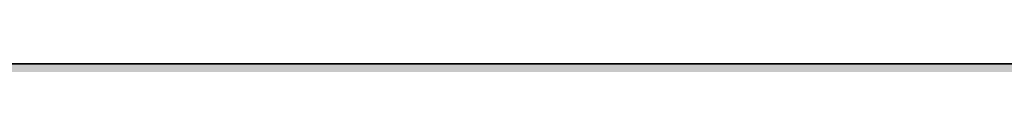
# Model space of a CAD drawing. Units: inches. Extents: x 2091 to 2899, y 967 to 2217.
# Tile 82 of 256: x 2245.941 to 2249.731, y 1099.919 to 1099.919. Entities that reach past the tile are written whole.
import ezdxf

# ---------------------------------------------------------------- set-up
doc = ezdxf.new("R2010")
doc.units = ezdxf.units.IN
doc.layers.add('A-WALL-PATT', color=141, linetype='Continuous', lineweight=13, true_color=0xadddf7)
doc.layers.add('L-SITE-WALL', color=7, linetype='Continuous', lineweight=35)

msp = doc.modelspace()

# ---------------------------------------------------------------- hatches: boundary and pattern name
at = {"layer": 'A-WALL-PATT'}
h = msp.add_hatch(color=256, dxfattribs=at)
h.dxf.hatch_style = 1
h.paths.add_polyline_path([(2212.1436, 1941.4191), (2387.6436, 1941.4191), (2387.6436, 1824.4191), (2392.1436, 1824.4191), (2392.1436, 1941.4191), (2609.6436, 1941.4191), (2609.6436, 1825.9191), (2614.1436, 1825.9191), (2614.1436, 1941.4191), (2794.1436, 1941.4191), (2794.1436, 1928.7622), (2803.1436, 1928.7622), (2803.1436, 2050.9191), (2203.1436, 2050.9191), (2203.1436, 1900.7579), (2212.1436, 1900.7579)])
h.paths.add_polyline_path([(2212.1436, 1945.9191), (2212.1436, 2041.9191), (2794.1436, 2041.9191), (2794.1436, 1945.9191), (2402.2482, 1945.9191), (2401.1024, 1945.7758), (2398.7024, 1945.7758)], flags=16)
h.paths.add_polyline_path([(2230.2299, 1948.0628), (2227.3499, 1949.5028), (2225.9099, 1951.9028), (2223.9899, 1952.8628), (2223.0299, 1955.2628), (2222.0699, 1959.5828), (2222.0699, 1963.4228), (2223.0299, 1965.6628), (2223.9899, 1965.3428), (2225.5859, 1963.8607), (2226.9115, 1964.9573), (2226.9489, 1965.9388), (2227.7783, 1966.9521), (2228.1999, 1968.8787), (2230.7099, 1964.8628), (2233.5899, 1966.3028), (2233.6073, 1966.3319), (2233.7727, 1964.9382), (2234.6338, 1963.6765), (2235.0299, 1963.9028), (2236.282, 1965.5724), (2235.9899, 1962.9428), (2237.9545, 1957.54), (2238.3899, 1957.9028), (2239.2159, 1960.3058), (2238.6546, 1966.385), (2238.6928, 1966.4381), (2238.8406, 1967.4997), (2238.7803, 1967.6875), (2238.8805, 1967.7868), (2238.6669, 1966.2518), (2239.2159, 1960.3058), (2238.3899, 1957.9028), (2236.9499, 1956.7028), (2234.5499, 1949.9828)], flags=0)
h.paths.add_polyline_path([(2278.012, 1948.0628), (2276.4964, 1947.8733), (2275.8498, 1947.6886), (2274.652, 1947.1028)], flags=0)
h.paths.add_polyline_path([(2269.852, 1955.7428), (2268.2762, 1956.6293), (2270.8673, 1956.3484), (2269.372, 1958.1428), (2268.715, 1959.1923), (2270.5698, 1958.7286), (2268.5807, 1961.9061), (2270.812, 1960.8919), (2270.812, 1963.4228), (2271.3933, 1964.7793), (2270.2918, 1966.1562), (2271.772, 1965.6628), (2272.1414, 1966.5248), (2273.9298, 1965.9286), (2275.6304, 1968.0543), (2276.3319, 1966.7219), (2276.5204, 1966.9521), (2276.942, 1968.8787), (2277.7343, 1967.6111), (2278.1399, 1969.4645), (2279.6591, 1967.0337), (2280.412, 1966.7828), (2280.9493, 1967.5888), (2281.6098, 1967.3686), (2282.1333, 1968.1538), (2282.3492, 1966.3334), (2282.3498, 1966.3326), (2283.4076, 1968.0954), (2283.7126, 1965.524), (2284.3202, 1964.6338), (2284.5118, 1964.8892), (2284.235, 1965.7048), (2284.5005, 1967.319), (2284.9079, 1965.4174), (2285.3963, 1966.0686), (2285.4328, 1966.2906), (2285.4733, 1966.1713), (2286.3539, 1967.3454), (2286.222, 1966.1582), (2287.6635, 1968.0802), (2287.714, 1968.4428), (2288.4816, 1969.0167), (2288.574, 1968.7289), (2288.9175, 1969.069), (2288.6068, 1966.8376), (2288.9287, 1963.3513), (2288.935, 1963.3568), (2288.9297, 1963.3404), (2289.0153, 1962.4139), (2290.1112, 1963.8751), (2290.1328, 1963.9426), (2290.2177, 1964.0171), (2290.1112, 1963.8751), (2289.1558, 1960.8916), (2288.594, 1959.2572), (2288.572, 1959.1028), (2289.532, 1960.5428), (2290.012, 1962.4628), (2290.1918, 1962.6427), (2289.7698, 1959.6886), (2286.8898, 1957.2886), (2284.4898, 1950.5686), (2283.3147, 1950.0463), (2283.292, 1949.9828), (2280.2901, 1948.6486), (2281.1298, 1948.6486), (2282.5698, 1948.1686), (2283.2047, 1948.0628), (2278.972, 1948.0628), (2276.092, 1949.5028), (2274.652, 1951.9028), (2272.732, 1952.8628)], flags=0)
h.paths.add_polyline_path([(2271.1589, 1958.0218), (2272.9698, 1955.8486), (2272.0098, 1960.1686), (2272.0098, 1964.0086), (2272.6244, 1965.4427), (2274.328, 1963.8607), (2275.6536, 1964.9573), (2275.6377, 1964.5391), (2277.4122, 1966.0069), (2277.033, 1965.1568), (2276.8299, 1964.9756), (2276.766, 1963.295), (2277.4496, 1962.6602), (2279.452, 1964.8628), (2282.332, 1966.3028), (2283.5298, 1966.8886), (2283.2945, 1966.7709), (2283.913, 1963.8847), (2284.8992, 1964.4483), (2284.732, 1962.9428), (2286.6966, 1957.54), (2287.132, 1957.9028), (2287.5419, 1959.0954), (2287.7794, 1958.4423), (2285.6827, 1956.6951), (2285.8765, 1959.7953), (2284.732, 1962.9428), (2284.8992, 1964.4483), (2283.913, 1963.8847), (2284.2238, 1962.4341), (2283.4244, 1963.6055), (2281.6098, 1962.5686), (2281.1298, 1960.1686), (2282.0898, 1956.3286), (2283.0498, 1952.9686), (2282.5698, 1950.5686), (2280.1698, 1948.6486), (2279.8833, 1948.7919), (2278.972, 1948.0628), (2278.972, 1949.0228), (2278.6723, 1949.3974), (2277.2898, 1950.0886), (2275.8498, 1952.4886), (2273.9298, 1953.4486), (2272.4898, 1954.8886), (2271.9216, 1954.8886), (2271.772, 1955.2628)], flags=0)
h.paths.add_polyline_path([(2311.9941, 1955.7428), (2312.0627, 1955.6742), (2312.0551, 1955.7085)], flags=0)
h.paths.add_polyline_path([(2331.9561, 1963.9518), (2333.3961, 1965.3918), (2331.0771, 1963.3568), (2330.9986, 1963.1115)], flags=0)
h.paths.add_polyline_path([(2310.5541, 1954.3028), (2307.0398, 1956.2799), (2310.7629, 1955.8763), (2312.4741, 1953.8228), (2313.4341, 1951.4228), (2315.3541, 1950.4628), (2316.7941, 1948.0628), (2317.4661, 1947.7268), (2319.3687, 1947.9646), (2317.7541, 1949.9828), (2317.5695, 1950.6105), (2316.7941, 1951.9028), (2314.8741, 1952.8628), (2313.9141, 1955.2628), (2311.5141, 1958.1428), (2309.3755, 1961.5592), (2311.5141, 1960.3371), (2311.5141, 1961.9828), (2310.6047, 1963.1196), (2311.7266, 1962.4785), (2312.4183, 1964.0926), (2312.256, 1964.2955), (2313.1941, 1963.9828), (2313.9141, 1965.6628), (2314.6468, 1965.4186), (2315.3541, 1966.3028), (2316.7941, 1967.7428), (2316.1574, 1966.9469), (2317.0341, 1965.2819), (2317.2226, 1965.5121), (2317.777, 1968.0458), (2318.4741, 1966.7219), (2318.6626, 1966.9521), (2319.0842, 1968.8787), (2321.207, 1965.4821), (2322.1614, 1966.9137), (2322.5541, 1966.7828), (2322.786, 1967.1306), (2322.8816, 1966.3243), (2323.312, 1965.7217), (2323.6513, 1965.8914), (2324.3965, 1967.1334), (2324.6569, 1964.9382), (2324.972, 1964.4766), (2325.3873, 1967.0015), (2325.9408, 1964.4183), (2327.2289, 1966.1358), (2327.1663, 1965.5724), (2328.0591, 1966.7628), (2328.2246, 1966.2475), (2329.668, 1967.6769), (2329.6646, 1967.6875), (2329.7648, 1967.7868), (2329.5511, 1966.2518), (2330.1001, 1960.3058), (2329.3328, 1958.0735), (2329.3131, 1957.9352), (2329.6341, 1958.2028), (2330.2341, 1959.1028), (2330.7141, 1961.0228), (2331.0341, 1961.3428), (2330.7141, 1959.1028), (2329.6341, 1958.2028), (2329.2741, 1957.6628), (2327.7121, 1956.3611), (2325.4341, 1949.9828), (2324.3338, 1949.4937), (2323.9941, 1948.5428), (2319.6741, 1946.6228), (2316.7941, 1948.0628), (2315.3541, 1950.4628), (2313.4341, 1951.4228)], flags=0)
h.paths.add_polyline_path([(2321.3357, 1947.952), (2321.1141, 1948.0628), (2321.1141, 1949.0228), (2319.1941, 1951.4228), (2316.7941, 1959.5828), (2316.6632, 1959.5828), (2315.3541, 1958.1428), (2314.3941, 1958.1428), (2313.1483, 1958.7091), (2312.9541, 1959.5828), (2312.9541, 1960.8919), (2315.8341, 1959.5828), (2316.6632, 1959.5828), (2317.3147, 1960.2994), (2315.0302, 1962.4207), (2316.3558, 1963.5173), (2316.3723, 1963.9516), (2316.4702, 1963.8607), (2317.7958, 1964.9573), (2317.7552, 1963.8897), (2319.1751, 1965.1568), (2319.4984, 1965.8814), (2321.1141, 1965.3428), (2323.2359, 1962.3724), (2325.6863, 1963.7726), (2325.5428, 1962.4806), (2325.1988, 1963.494), (2324.4785, 1963.0824), (2324.926, 1960.9941), (2324.0781, 1962.2365), (2322.4148, 1961.286), (2322.0741, 1959.5828), (2323.0341, 1955.7428), (2323.9941, 1952.3828), (2323.5141, 1949.9828), (2322.1427, 1948.8856), (2322.0741, 1948.5428)], flags=0)
h.paths.add_polyline_path([(2320.2075, 1963.3375), (2320.1541, 1963.4228), (2320.3941, 1963.5428)], flags=0)
h.paths.add_polyline_path([(2353.8505, 1965.8105), (2354.0305, 1965.7505), (2354.3305, 1966.4505), (2354.3305, 1966.9305)], flags=0)
h.paths.add_polyline_path([(2359.0206, 1969.0264), (2359.0984, 1968.9019), (2359.2335, 1969.5195), (2359.2335, 1969.9995)], flags=0)
h.paths.add_polyline_path([(2358.2567, 1966.6817), (2357.9836, 1966.348), (2358.2113, 1966.1462), (2358.4105, 1966.3896)], flags=0)
h.paths.add_polyline_path([(2357.7685, 1966.0588), (2357.7322, 1965.105), (2357.751, 1965.1206), (2357.7695, 1965.6065), (2357.7695, 1966.0578)], flags=0)
h.paths.add_polyline_path([(2359.1115, 1965.3045), (2359.1115, 1964.8245), (2359.8445, 1966.4675), (2359.8445, 1966.9475)], flags=0)
h.paths.add_polyline_path([(2360.2237, 1966.6214), (2360.6985, 1969.3625), (2360.6985, 1969.8425), (2360.2105, 1967.0255), (2360.2105, 1966.6425)], flags=0)
h.paths.add_polyline_path([(2363.4505, 1967.8905), (2363.4505, 1968.3705), (2362.4905, 1966.9305), (2362.656, 1966.6988)], flags=0)
h.paths.add_polyline_path([(2364.4755, 1966.0788), (2365.8505, 1968.3705), (2365.8505, 1968.8505), (2364.428, 1966.4796)], flags=0)
h.paths.add_polyline_path([(2366.3135, 1965.8525), (2366.3667, 1965.6958), (2366.8025, 1968.3455), (2366.8025, 1968.8255)], flags=0)
h.paths.add_polyline_path([(2367.1653, 1965.8035), (2367.2905, 1966.9305), (2367.2905, 1967.4105), (2367.1027, 1965.7201)], flags=0)
h.paths.add_polyline_path([(2370.0365, 1959.9735), (2371.0135, 1963.0245), (2371.0135, 1963.5045), (2370.0365, 1960.4535)], flags=0)
h.paths.add_polyline_path([(2371.6105, 1960.2105), (2372.5705, 1961.6505), (2372.5705, 1962.1305), (2371.8025, 1960.9785)], flags=0)
h.paths.add_polyline_path([(2350.8737, 1956.0051), (2351.9305, 1955.8905), (2354.4905, 1953.3305), (2353.8505, 1954.9305), (2351.4505, 1957.8105), (2347.9355, 1963.4255), (2347.9355, 1963.9055), (2351.4505, 1958.2905), (2353.7051, 1955.585), (2352.8905, 1959.2505), (2352.8905, 1959.7305), (2352.8905, 1961.9248), (2356.7305, 1959.7305), (2358.4545, 1961.6268), (2354.8105, 1965.0105), (2355.0309, 1965.2859), (2358.6911, 1961.8871), (2361.5305, 1965.0105), (2364.3765, 1966.4335), (2364.5244, 1965.1869), (2365.4545, 1963.8242), (2365.8811, 1964.068), (2365.3705, 1966.4505), (2365.3705, 1966.9305), (2366.8105, 1960.2105), (2366.8105, 1959.7305), (2366.3887, 1952.9814), (2367.7705, 1956.8505), (2368.6412, 1957.5761), (2366.8105, 1962.6105), (2366.8105, 1963.0905), (2368.7752, 1957.6877), (2369.2105, 1958.0505), (2370.0016, 1960.3519), (2369.4752, 1966.0527), (2369.5135, 1966.1058), (2369.5142, 1966.1109), (2369.4752, 1966.5327), (2369.5135, 1966.5858), (2369.6146, 1967.3126), (2369.1825, 1968.6585), (2369.1825, 1969.1385), (2369.601, 1967.8352), (2369.7012, 1967.9345), (2369.7179, 1968.0547), (2370.1452, 1968.3741), (2369.7787, 1968.0112), (2369.7012, 1967.4545), (2370.4682, 1968.214), (2369.6749, 1967.2658), (2369.5142, 1966.1109), (2370.0365, 1960.4535), (2370.0365, 1959.9735), (2369.4418, 1958.2432), (2370.6505, 1959.2505), (2371.0458, 1962.0176), (2371.1305, 1962.1305), (2370.6505, 1958.7705), (2367.7705, 1956.3705), (2365.3705, 1949.6505), (2362.0791, 1948.1876), (2363.4505, 1947.7305), (2361.0505, 1947.7305), (2360.0905, 1947.7305), (2357.1039, 1947.3572), (2360.0905, 1948.2105), (2358.1705, 1949.1705), (2356.7305, 1951.5705), (2354.8105, 1952.5305), (2351.9305, 1955.4105)], flags=0)
h.paths.add_polyline_path([(2361.0505, 1948.6905), (2359.1305, 1951.0905), (2356.7305, 1959.2505), (2355.7705, 1959.2505), (2352.8905, 1960.5596), (2352.8905, 1961.4448), (2355.8905, 1959.7305), (2356.7305, 1959.7305), (2356.8372, 1959.3678), (2361.5305, 1964.5305), (2363.2484, 1965.3894), (2364.9253, 1963.0418), (2362.4905, 1961.6505), (2362.0639, 1959.5172), (2362.9705, 1955.8905), (2363.9305, 1952.5305), (2363.9305, 1952.0505), (2363.4505, 1949.6505), (2361.0505, 1947.7305)], flags=0)
h.paths.add_polyline_path([(2359.1305, 1951.5705), (2359.2905, 1951.3705), (2361.0505, 1954.4505), (2361.0505, 1954.9305)], flags=0)
h.paths.add_polyline_path([(2357.2195, 1966.5455), (2356.7925, 1968.8145), (2356.7925, 1969.2945), (2357.2195, 1967.0255)], flags=0)
h.paths.add_polyline_path([(2361.0505, 1954.4505), (2361.5305, 1958.7705), (2361.5305, 1959.2505), (2361.0505, 1954.9305)], flags=0)
h.paths.add_polyline_path([(2402.5483, 1948.4861), (2402.3024, 1948.4158), (2402.5904, 1948.4158)], flags=0)
h.paths.add_polyline_path([(2394.1424, 1956.0958), (2395.6851, 1954.5532), (2396.7205, 1953.9707), (2396.0624, 1955.6158), (2395.2414, 1956.6011), (2395.8789, 1956.4417), (2395.1024, 1959.9358), (2395.1024, 1963.7758), (2396.0624, 1966.0158), (2397.0224, 1965.6958), (2398.6185, 1964.2138), (2399.9441, 1965.3103), (2399.9814, 1966.2918), (2400.8109, 1967.3052), (2401.2325, 1969.2317), (2403.5379, 1965.543), (2403.942, 1967.3893), (2404.7024, 1967.1358), (2405.4603, 1966.0748), (2406.6224, 1966.6558), (2406.6399, 1966.6849), (2406.8052, 1965.2912), (2406.9257, 1965.1147), (2407.3424, 1964.9758), (2407.8743, 1965.7737), (2408.1691, 1964.3981), (2409.3146, 1965.9254), (2409.2175, 1965.0511), (2409.4452, 1963.1312), (2410.3064, 1961.8695), (2410.7024, 1962.0958), (2411.4423, 1963.0823), (2411.1654, 1963.8978), (2411.6164, 1966.6398), (2411.7254, 1966.7911), (2411.8732, 1967.8527), (2411.8129, 1968.0405), (2411.9131, 1968.1398), (2411.6994, 1966.6048), (2412.2484, 1960.6588), (2413.2254, 1963.7098), (2414.3779, 1964.7212), (2414.5132, 1965.6927), (2414.4529, 1965.8805), (2414.5531, 1965.9798), (2414.3779, 1964.7212), (2414.5198, 1964.8457), (2414.3654, 1964.6311), (2414.3394, 1964.4448), (2414.8884, 1958.4988), (2414.0624, 1956.0958), (2412.6224, 1954.8958), (2410.1714, 1948.0329), (2410.0167, 1948.0844), (2405.9024, 1946.2558), (2405.9024, 1947.2158), (2405.2043, 1948.0886), (2404.2224, 1948.4158), (2403.2624, 1948.4158), (2400.3824, 1949.8558), (2399.6624, 1951.0558), (2397.9824, 1952.7358), (2397.0224, 1953.2158), (2395.6851, 1954.5532), (2392.6568, 1956.2569)], flags=0)
h.paths.add_polyline_path([(2409.0857, 1964.4074), (2409.1304, 1964.2757), (2409.2624, 1964.4958)], flags=0)
h.paths.add_polyline_path([(2397.7424, 1961.6158), (2398.7024, 1963.8558), (2399.6624, 1963.5358), (2401.4266, 1965.741), (2401.7914, 1966.5588), (2402.0714, 1965.0708), (2402.8355, 1964.3934), (2403.2624, 1964.9149), (2403.3381, 1964.7711), (2402.6155, 1963.9762), (2402.4986, 1960.9022), (2403.543, 1959.9325), (2404.4132, 1960.8897), (2404.7024, 1962.3358), (2407.9163, 1964.1724), (2409.5202, 1961.9269), (2410.9871, 1957.893), (2411.4224, 1958.2558), (2412.048, 1960.0756), (2412.4103, 1959.0791), (2411.6756, 1958.4668), (2411.6624, 1958.2558), (2411.6261, 1958.4255), (2409.9824, 1957.0558), (2407.5824, 1950.3358), (2403.2624, 1948.4158), (2403.2624, 1949.3758), (2401.3424, 1951.7758), (2399.4165, 1958.324), (2397.7424, 1959.0849), (2397.7424, 1959.9701), (2397.1024, 1960.3358), (2397.7424, 1960.0449)], flags=0)
h.paths.add_polyline_path([(2405.9024, 1952.9758), (2405.9504, 1953.4078), (2406.0167, 1953.1758)], flags=0)
h.paths.add_polyline_path([(2449.8178, 1967.114), (2449.7523, 1967.1358), (2449.7937, 1967.0779)], flags=0)
h.paths.add_polyline_path([(2451.6977, 1966.6181), (2451.7409, 1966.6901), (2451.6921, 1966.6657)], flags=0)
h.paths.add_polyline_path([(2454.3436, 1965.7376), (2455.7523, 1967.6158), (2455.9923, 1968.0958), (2454.3645, 1965.9254)], flags=0)
h.paths.add_polyline_path([(2457.5473, 1968.8638), (2457.7873, 1969.3438), (2457.0543, 1968.7958), (2457.0076, 1968.4603)], flags=0)
h.paths.add_polyline_path([(2456.9218, 1967.8567), (2456.8022, 1968.229), (2456.723, 1967.6598)], flags=0)
h.paths.add_polyline_path([(2457.3023, 1967.3768), (2457.5423, 1967.8568), (2456.8103, 1966.8398), (2456.7405, 1966.7002), (2456.749, 1966.6081)], flags=0)
h.paths.add_polyline_path([(2458.2753, 1963.7098), (2458.1553, 1963.3352), (2460.3543, 1965.2648), (2460.5943, 1965.7448)], flags=0)
h.paths.add_polyline_path([(2458.3923, 1962.8158), (2458.3641, 1962.6182), (2459.5923, 1964.2558), (2459.8323, 1964.7358)], flags=0)
h.paths.add_polyline_path([(2459.3523, 1962.8158), (2459.2723, 1962.4958), (2460.0723, 1963.2958), (2460.3123, 1963.7758)], flags=0)
h.paths.add_polyline_path([(2458.6803, 1960.6078), (2458.6323, 1960.4158), (2459.5923, 1961.8558), (2459.8323, 1962.3358)], flags=0)
h.paths.add_polyline_path([(2437.8382, 1956.2427), (2439.1923, 1956.0958), (2441.3523, 1953.9358), (2440.8723, 1955.1358), (2438.4723, 1958.0158), (2438.0716, 1958.656), (2438.7123, 1958.4958), (2440.6396, 1956.1831), (2439.9123, 1959.4558), (2439.9123, 1963.2958), (2441.3523, 1966.6558), (2441.5923, 1967.1358), (2441.1123, 1966.0158), (2442.0723, 1965.6958), (2443.989, 1968.0917), (2444.2413, 1966.7508), (2444.9168, 1966.1519), (2445.6766, 1967.0801), (2446.2553, 1969.7248), (2446.4953, 1970.2048), (2446.2824, 1969.2317), (2447.3627, 1967.5033), (2447.7203, 1969.5678), (2447.9603, 1970.0478), (2447.4855, 1967.3068), (2448.7923, 1965.2158), (2448.4723, 1964.8638), (2448.5523, 1964.7358), (2451.4521, 1966.1857), (2451.6151, 1964.8112), (2452.3079, 1963.7962), (2453.2345, 1964.3257), (2454.0723, 1960.4158), (2453.6287, 1953.3177), (2454.7923, 1956.5758), (2455.0323, 1957.0558), (2455.7188, 1957.6279), (2453.8323, 1962.8158), (2453.941, 1963.7936), (2453.3353, 1965.5778), (2453.8243, 1968.5508), (2454.0643, 1969.0308), (2453.5753, 1966.0578), (2454.0403, 1964.6879), (2453.8323, 1962.8158), (2455.7188, 1957.6279), (2456.3672, 1958.1682), (2457.0583, 1960.1788), (2457.2983, 1960.6588), (2456.4723, 1958.2558), (2457.7177, 1959.2937), (2457.6723, 1958.9758), (2454.89, 1956.6572), (2453.6141, 1953.0849), (2453.5923, 1952.7358), (2453.3523, 1952.2558), (2453.3596, 1952.3722), (2452.6323, 1950.3358), (2452.3923, 1949.8558), (2449.2038, 1948.4387), (2450.7123, 1947.9358), (2448.0723, 1947.9358), (2447.1123, 1947.9358), (2444.5523, 1947.6158), (2447.1996, 1948.3722), (2445.1923, 1949.3758), (2443.7523, 1951.7758), (2441.8323, 1952.7358), (2438.9523, 1955.6158)], flags=0)
h.paths.add_polyline_path([(2443.9923, 1959.9358), (2444.0403, 1959.7726), (2444.1216, 1959.862)], flags=0)
h.paths.add_polyline_path([(2442.9123, 1959.9358), (2443.0323, 1959.9358), (2442.4457, 1960.2025)], flags=0)
h.paths.add_polyline_path([(2444.9829, 1965.0197), (2445.2793, 1965.2648), (2445.5193, 1965.7448), (2444.994, 1965.3103)], flags=0)
h.paths.add_polyline_path([(2446.1333, 1965.0298), (2446.3304, 1965.4715), (2444.9703, 1964.2578), (2444.7303, 1963.7778)], flags=0)
h.paths.add_polyline_path([(2442.7923, 1959.4558), (2443.7523, 1959.4558), (2446.1523, 1951.2958), (2446.4123, 1951.7508), (2446.3923, 1951.7758), (2448.0806, 1954.7303), (2448.5523, 1958.9758), (2441.8323, 1965.2158), (2442.1549, 1965.6191), (2448.7923, 1959.4558), (2448.3123, 1955.1358), (2448.0723, 1954.6558), (2446.4123, 1951.7508), (2448.3123, 1949.3758), (2448.3123, 1948.4158), (2450.5409, 1950.1987), (2450.9523, 1952.2558), (2449.9923, 1955.6158), (2449.0323, 1959.4558), (2449.5123, 1961.8558), (2449.7523, 1962.3358), (2449.6749, 1961.9487), (2452.9945, 1963.8457), (2453.0644, 1963.5194), (2452.8846, 1963.7829), (2449.6749, 1961.9487), (2449.2723, 1959.9358), (2450.2323, 1956.0958), (2451.1923, 1952.7358), (2450.7123, 1950.3358), (2450.4723, 1949.8558), (2448.0723, 1947.9358), (2448.0723, 1948.5358), (2445.4323, 1949.8558), (2443.9923, 1952.2558), (2442.0723, 1953.2158), (2441.1123, 1955.6158), (2440.1523, 1959.9358), (2440.1523, 1960.6558)], flags=0)
h.paths.add_polyline_path([(2456.6923, 1966.9858), (2457.6083, 1968.0808), (2457.8483, 1968.5608), (2456.9323, 1967.4658)], flags=0)
h.paths.add_polyline_path([(2489.8966, 1966.5802), (2489.9429, 1966.1893), (2490.7475, 1967.5302), (2491.3191, 1968.9512)], flags=0)
h.paths.add_polyline_path([(2473.5625, 1956.4071), (2477.14, 1956.0193), (2476.9553, 1956.2408), (2475.108, 1957.2801), (2476.3475, 1956.9702), (2475.1869, 1958.8242), (2476.9191, 1958.3912), (2475.4116, 1960.7993), (2477.7875, 1959.7193), (2477.7875, 1962.2502), (2477.6374, 1962.4379), (2477.8226, 1962.3321), (2478.3591, 1963.5841), (2478.3591, 1963.6712), (2477.3243, 1964.9646), (2478.7148, 1964.5011), (2479.3191, 1965.9112), (2480.2791, 1965.5912), (2481.784, 1967.4722), (2482.1165, 1965.7052), (2482.8806, 1965.0278), (2483.2093, 1965.4294), (2483.2202, 1965.7151), (2483.0759, 1965.989), (2483.7118, 1966.7658), (2484.1305, 1968.6792), (2484.7021, 1970.1002), (2484.4892, 1969.1271), (2486.5029, 1965.9051), (2487.3875, 1965.6102), (2488.1534, 1966.7591), (2488.717, 1965.9701), (2489.2001, 1966.2116), (2489.3307, 1965.111), (2490.3939, 1963.6225), (2490.6608, 1963.775), (2490.4939, 1964.5536), (2490.9231, 1963.9248), (2491.3191, 1964.1512), (2491.3334, 1964.1702), (2491.2105, 1964.5322), (2491.2818, 1964.9655), (2491.4258, 1964.2934), (2494.0765, 1967.8276), (2494.4979, 1966.5149), (2494.5982, 1966.6142), (2494.6895, 1967.2702), (2495.1067, 1967.5822), (2495.1298, 1967.7481), (2495.0696, 1967.9359), (2495.1698, 1968.0351), (2495.0318, 1967.0436), (2495.7538, 1967.7587), (2494.9821, 1966.6864), (2494.9561, 1966.5002), (2495.479, 1960.8369), (2495.9105, 1962.1842), (2496.4821, 1963.6052), (2496.0727, 1962.3266), (2496.7689, 1962.9375), (2496.5991, 1962.7112), (2496.1191, 1959.3512), (2496.7329, 1960.2718), (2496.9875, 1961.2902), (2497.5591, 1962.7112), (2497.0791, 1960.7912), (2496.5075, 1959.3702), (2495.5475, 1957.9302), (2492.7588, 1955.6064), (2490.8391, 1950.2312), (2490.2675, 1948.8102), (2485.9475, 1946.8902), (2483.0675, 1948.3302), (2481.6275, 1950.7302), (2479.7075, 1951.6902), (2476.8275, 1954.5702)], flags=0)
h.paths.add_polyline_path([(2485.577, 1948.3134), (2485.5591, 1948.3112), (2485.5788, 1948.3112)], flags=0)
h.paths.add_polyline_path([(2478.6451, 1954.5512), (2478.109, 1956.9633), (2479.3191, 1955.5112), (2480.2791, 1953.1112), (2482.1991, 1952.1512), (2483.6391, 1949.7512), (2486.5191, 1948.3112), (2486.5191, 1949.2712), (2484.7393, 1951.4959), (2484.0275, 1950.2502), (2481.6275, 1958.4102), (2482.3751, 1959.2327), (2482.1991, 1959.8312), (2483.1976, 1960.9295), (2479.7075, 1964.1702), (2480.6034, 1965.2901), (2481.8752, 1964.1091), (2482.6664, 1964.7636), (2482.6154, 1963.4218), (2482.9892, 1963.0747), (2484.0085, 1963.9842), (2484.6836, 1965.4975), (2484.5801, 1965.4052), (2485.3573, 1967.1471), (2485.1206, 1965.7812), (2486.4275, 1963.6902), (2488.1454, 1964.5492), (2489.8223, 1962.2016), (2490.7475, 1962.7302), (2491.9997, 1964.3998), (2492.076, 1965.0873), (2492.2129, 1964.6841), (2492.4854, 1965.0474), (2492.2791, 1963.1912), (2494.2438, 1957.7884), (2494.5625, 1958.054), (2494.9335, 1959.1332), (2495.5051, 1960.5542), (2494.6791, 1958.1512), (2494.1075, 1956.7302), (2494.5625, 1958.054), (2493.4085, 1957.0923), (2491.7075, 1961.7702), (2491.9997, 1964.3998), (2490.7475, 1962.7302), (2487.712, 1960.9957), (2487.4791, 1959.8312), (2488.4391, 1955.9912), (2489.3991, 1952.6312), (2488.9191, 1950.2312), (2488.5769, 1949.9574), (2488.3475, 1948.8102), (2487.6517, 1948.2536), (2487.4791, 1948.3112), (2486.5191, 1948.3112), (2483.6391, 1949.7512), (2482.1991, 1952.1512), (2480.2791, 1953.1112), (2478.8391, 1954.5512)], flags=0)
h.paths.add_polyline_path([(2526.6483, 1966.9875), (2526.5173, 1967.0312), (2526.6001, 1966.9153)], flags=0)
h.paths.add_polyline_path([(2528.4706, 1966.4467), (2528.5745, 1966.6197), (2528.4571, 1966.561)], flags=0)
h.paths.add_polyline_path([(2534.1333, 1967.4962), (2534.1567, 1967.5428), (2534.0598, 1967.4083)], flags=0)
h.paths.add_polyline_path([(2536.1619, 1964.0506), (2535.1573, 1962.7112), (2535.1009, 1962.3159), (2536.1173, 1963.6712), (2536.4205, 1964.2775)], flags=0)
h.paths.add_polyline_path([(2535.1573, 1959.8312), (2536.1173, 1961.2712), (2536.5973, 1962.2312), (2535.2533, 1960.2152)], flags=0)
h.paths.add_polyline_path([(2513.249, 1956.2848), (2516.2212, 1955.9626), (2514.9973, 1957.4312), (2514.1958, 1958.7115), (2515.4773, 1958.3912), (2516.9319, 1956.6457), (2516.4373, 1958.8712), (2516.4373, 1962.7112), (2516.8727, 1963.727), (2515.3464, 1965.6348), (2517.3973, 1964.9512), (2517.8773, 1966.0712), (2518.3573, 1967.0312), (2517.8773, 1965.9112), (2518.8373, 1965.5912), (2520.4866, 1967.6527), (2520.7663, 1966.1662), (2521.5304, 1965.4887), (2521.7814, 1965.7954), (2521.8009, 1966.3073), (2521.4778, 1966.9209), (2521.2463, 1967.1262), (2521.1777, 1967.4909), (2521.4778, 1966.9209), (2522.0104, 1966.4487), (2522.2574, 1966.7504), (2522.7803, 1969.1402), (2523.2603, 1970.1002), (2523.0474, 1969.1271), (2524.6731, 1966.5259), (2526.0373, 1966.0712), (2526.7952, 1965.0101), (2527.9771, 1965.601), (2528.1401, 1964.2266), (2528.6646, 1963.4582), (2529.3886, 1963.8719), (2529.3297, 1964.147), (2529.4813, 1963.9248), (2529.8773, 1964.1512), (2529.984, 1964.2934), (2529.7891, 1965.2032), (2530.0624, 1964.3979), (2532.8025, 1968.0513), (2533.1478, 1966.9759), (2533.248, 1967.0751), (2533.3393, 1967.7312), (2533.6728, 1967.9805), (2533.728, 1968.0351), (2533.5143, 1966.5002), (2534.0247, 1960.9725), (2534.5603, 1962.6452), (2535.0403, 1963.6052), (2534.0633, 1960.5542), (2533.2373, 1958.1512), (2534.2882, 1959.0268), (2534.1973, 1958.3912), (2531.5126, 1956.1539), (2529.3973, 1950.2312), (2528.9173, 1949.2712), (2526.4488, 1948.174), (2527.4773, 1947.8312), (2530.3573, 1947.3512), (2524.5973, 1947.3512), (2521.7173, 1948.7912), (2520.2773, 1951.1912), (2518.3573, 1952.1512), (2515.4773, 1955.0312)], flags=0)
h.paths.add_polyline_path([(2523.9348, 1967.1903), (2523.6195, 1966.4837), (2523.7705, 1966.2421)], flags=0)
h.paths.add_polyline_path([(2518.8373, 1953.1112), (2517.8773, 1955.5112), (2516.885, 1959.9768), (2516.9173, 1959.9621), (2516.9173, 1962.0254), (2520.7573, 1959.8312), (2522.0249, 1961.2255), (2518.3573, 1964.6312), (2519.0026, 1965.4377), (2520.4334, 1964.1091), (2521.3011, 1964.8269), (2521.2452, 1963.3553), (2525.6383, 1959.276), (2526.0373, 1961.2712), (2529.3973, 1963.1912), (2530.6495, 1964.8607), (2530.6647, 1964.9976), (2530.692, 1964.9173), (2531.0878, 1965.4451), (2530.946, 1964.1689), (2530.692, 1964.9173), (2529.3973, 1963.1912), (2526.3625, 1961.457), (2526.0373, 1959.8312), (2526.9973, 1955.9912), (2527.9573, 1952.6312), (2527.4773, 1950.2312), (2527.1345, 1949.9569), (2526.9739, 1949.1541), (2526.6973, 1949.0312), (2524.5973, 1947.3512), (2524.5973, 1948.3112), (2524.2773, 1948.7112), (2522.1973, 1949.7512), (2520.7573, 1952.1512)], flags=0)
h.paths.add_polyline_path([(2520.2773, 1958.8712), (2520.8533, 1959.5048), (2523.1573, 1951.6712), (2524.6139, 1954.2201), (2524.5973, 1954.0712), (2522.6773, 1950.7112)], flags=0)
h.paths.add_polyline_path([(2559.3709, 1966.3112), (2559.3984, 1966.3249), (2559.4019, 1966.3453)], flags=0)
h.paths.add_polyline_path([(2549.7709, 1957.1912), (2552.6509, 1954.3112), (2552.134, 1955.6035), (2550.6109, 1957.4312), (2547.0959, 1963.0462), (2545.7759, 1965.2062), (2549.2909, 1959.5912), (2551.6909, 1956.7112), (2550.7929, 1960.7521), (2550.7309, 1960.7803), (2550.7309, 1964.8712), (2551.6909, 1967.1112), (2552.6509, 1966.7912), (2554.247, 1965.3091), (2555.0343, 1965.9603), (2555.5817, 1966.6446), (2555.6099, 1967.3872), (2556.4394, 1968.4005), (2556.861, 1970.3271), (2559.3709, 1966.3112), (2560.6909, 1964.1512), (2562.4088, 1965.0101), (2561.6509, 1966.0712), (2560.3309, 1968.2312), (2561.7585, 1966.2325), (2562.3472, 1967.1156), (2562.4337, 1966.3866), (2563.1278, 1965.3696), (2563.5709, 1965.5912), (2563.5884, 1965.6202), (2563.3625, 1967.5235), (2563.7225, 1965.8438), (2565.06, 1968.073), (2564.7329, 1965.1287), (2565.1176, 1963.3334), (2567.4446, 1966.4361), (2567.3156, 1967.8333), (2567.3538, 1967.8864), (2567.5016, 1968.9481), (2567.4413, 1969.1359), (2567.5416, 1969.2351), (2567.3279, 1967.7002), (2567.8769, 1961.7542), (2568.7467, 1964.4703), (2568.6356, 1965.6733), (2568.6738, 1965.7264), (2568.8216, 1966.7881), (2568.7613, 1966.9759), (2568.8616, 1967.0751), (2568.6479, 1965.5402), (2568.7261, 1964.693), (2568.8539, 1964.8052), (2568.7467, 1964.4703), (2568.8172, 1963.7063), (2568.9709, 1963.9112), (2568.8661, 1963.1773), (2569.1969, 1959.5942), (2568.3709, 1957.1912), (2566.9309, 1955.9912), (2564.6203, 1949.5214), (2564.6509, 1949.5112), (2564.6166, 1949.5112), (2564.5309, 1949.2712), (2560.2109, 1947.3512), (2557.3309, 1948.7912), (2556.0452, 1950.934), (2556.0109, 1950.9512), (2555.8566, 1951.2083), (2553.9709, 1952.1512), (2551.0909, 1955.0312), (2546.6501, 1957.5295)], flags=0)
h.paths.add_polyline_path([(2567.0258, 1959.3302), (2567.035, 1959.3049), (2567.0509, 1959.3512)], flags=0)
h.paths.add_polyline_path([(2551.9683, 1962.5184), (2553.0109, 1964.9512), (2553.9709, 1964.6312), (2555.567, 1963.1491), (2556.8926, 1964.2456), (2556.9299, 1965.2272), (2557.144, 1965.4887), (2556.4201, 1966.1306), (2556.3914, 1966.105), (2556.3799, 1966.1662), (2556.4201, 1966.1306), (2556.9519, 1966.6052), (2557.0921, 1966.9195), (2557.5709, 1966.0102), (2557.7594, 1966.2405), (2557.4179, 1964.6802), (2556.8926, 1964.2456), (2556.8071, 1961.9976), (2560.6909, 1958.3912), (2560.6355, 1957.8927), (2560.8109, 1957.1912), (2561.7709, 1953.8312), (2561.2909, 1951.4312), (2559.1104, 1949.6868), (2559.1565, 1949.6292), (2563.0265, 1951.3492), (2562.6109, 1949.2712), (2560.2109, 1947.3512), (2560.2109, 1948.3112), (2559.2509, 1949.5112), (2558.8909, 1949.5112), (2558.8909, 1949.9612), (2558.2909, 1950.7112), (2558.0537, 1951.5177), (2556.9709, 1952.8712), (2555.0679, 1959.3415), (2552.0509, 1961.0654), (2552.0509, 1962.4712)], flags=0)
h.paths.add_polyline_path([(2588.33, 1958.3912), (2588.6102, 1958.111), (2588.5534, 1958.3669)], flags=0)
h.paths.add_polyline_path([(2594.7455, 1950.4931), (2593.9575, 1953.172), (2593.13, 1954.5512), (2591.21, 1955.5112), (2590.25, 1957.9112), (2588.309, 1960.2404), (2586.1773, 1961.2093), (2587.85, 1960.7912), (2587.2534, 1961.7442), (2588.4413, 1961.0654), (2588.4413, 1962.6555), (2588.4217, 1962.6653), (2588.4413, 1962.7112), (2586.914, 1964.6203), (2588.8771, 1963.728), (2589.29, 1964.6915), (2589.29, 1966.0712), (2590.25, 1968.3112), (2591.21, 1967.9912), (2592.8061, 1966.5091), (2594.1317, 1967.6056), (2594.169, 1968.5872), (2594.9985, 1969.6005), (2595.4201, 1971.5271), (2597.93, 1967.5112), (2600.81, 1968.9512), (2600.8275, 1968.9802), (2600.9928, 1967.5866), (2601.854, 1966.3248), (2602.1071, 1966.4695), (2602.2364, 1967.2551), (2602.3567, 1966.6934), (2603.5022, 1968.2207), (2603.21, 1965.5912), (2605.1747, 1960.1884), (2605.5069, 1960.4652), (2605.026, 1965.6733), (2605.0642, 1965.7264), (2605.212, 1966.7881), (2605.1517, 1966.9759), (2605.252, 1967.0751), (2605.3433, 1967.7312), (2605.9529, 1968.1869), (2605.8748, 1969.0333), (2605.913, 1969.0864), (2606.0608, 1970.1481), (2606.0005, 1970.3359), (2606.1007, 1970.4351), (2605.887, 1968.9002), (2606.436, 1962.9542), (2605.61, 1960.5512), (2605.997, 1960.8737), (2606.5643, 1962.6452), (2608.2415, 1964.1169), (2608.01, 1963.1912), (2607.05, 1961.7512), (2606.6315, 1961.4024), (2606.2013, 1958.3912), (2603.3213, 1955.9912), (2600.9213, 1949.2712), (2596.6013, 1947.3512), (2593.7213, 1948.7912), (2592.8573, 1950.2312), (2592.65, 1950.2312)], flags=0)
h.paths.add_polyline_path([(2596.6013, 1947.3512), (2596.6013, 1948.3112), (2594.6813, 1950.7112), (2596.155, 1953.29), (2595.53, 1954.0712), (2593.1992, 1961.996), (2592.6513, 1962.5047), (2591.7802, 1963.0025), (2593.283, 1964.2456), (2593.3203, 1965.2272), (2594.1498, 1966.2405), (2594.5714, 1968.1671), (2596.1827, 1965.589), (2596.9513, 1966.4345), (2598.0413, 1966.0712), (2598.7992, 1965.0101), (2599.9613, 1965.5912), (2599.9788, 1965.6202), (2600.1441, 1964.2266), (2601.0053, 1962.9648), (2601.4013, 1963.1912), (2602.6535, 1964.8607), (2602.3613, 1962.2312), (2603.7927, 1958.2947), (2601.9776, 1953.2124), (2601.9462, 1952.7095), (2599.4688, 1951.6084), (2599.0013, 1949.2712)], flags=0)
h.paths.add_polyline_path([(2597.5613, 1958.8712), (2597.671, 1959.4194), (2597.5951, 1958.7362)], flags=0)
h.paths.add_polyline_path([(2623.6663, 1961.2544), (2625.5192, 1960.7912), (2624.9655, 1961.6755), (2627.1992, 1960.6603), (2627.1992, 1961.1512), (2626.9592, 1962.2312), (2626.9592, 1963.4912), (2625.5823, 1965.2122), (2626.9592, 1964.4254), (2626.9592, 1965.8312), (2626.8692, 1965.8612), (2627.9192, 1968.3112), (2628.8792, 1967.9912), (2630.4752, 1966.5091), (2631.8008, 1967.6056), (2631.8382, 1968.5872), (2632.6676, 1969.6005), (2633.0892, 1971.5271), (2635.5992, 1967.5112), (2638.4792, 1968.9512), (2638.4966, 1968.9802), (2638.662, 1967.5866), (2639.1763, 1966.833), (2639.7802, 1967.8396), (2640.0258, 1966.6934), (2641.1713, 1968.2207), (2640.8792, 1965.5912), (2641.1143, 1964.9446), (2641.4113, 1965.3407), (2641.3081, 1964.4116), (2642.8438, 1960.1884), (2643.2792, 1960.5512), (2644.0847, 1962.8947), (2643.7839, 1966.1533), (2643.8068, 1966.1852), (2643.6007, 1968.4181), (2643.5228, 1968.6606), (2643.7299, 1970.1481), (2643.6696, 1970.3359), (2643.7698, 1970.4351), (2643.5562, 1968.9002), (2643.6007, 1968.4181), (2643.9096, 1967.4559), (2644.0098, 1967.5551), (2643.8117, 1966.1321), (2644.1052, 1962.9542), (2644.2388, 1961.3508), (2644.7192, 1961.7512), (2645.0329, 1962.2217), (2645.3222, 1963.1252), (2646.0764, 1963.787), (2645.0329, 1962.2217), (2644.3452, 1960.0742), (2643.5192, 1957.6712), (2642.0792, 1956.4712), (2639.7196, 1949.8644), (2639.8755, 1949.8384), (2635.3592, 1947.8312), (2632.4792, 1949.2712), (2631.0392, 1951.6712), (2629.1192, 1952.6312), (2628.1592, 1955.0312), (2625.7592, 1957.9112)], flags=0)
h.paths.add_polyline_path([(2627.8163, 1956.574), (2627.3737, 1958.5657), (2626.3763, 1959.7626), (2627.1992, 1959.3512), (2627.3737, 1958.5657), (2627.9192, 1957.9112), (2628.8792, 1955.5112), (2630.7992, 1954.5512), (2632.2392, 1952.1512), (2633.315, 1951.6132), (2631.0392, 1959.3512), (2631.4978, 1959.8557), (2630.7992, 1962.2312), (2631.4499, 1962.9469), (2630.7152, 1963.6291), (2632.0408, 1964.7256), (2632.0782, 1965.7072), (2632.2922, 1965.9687), (2631.7053, 1966.4891), (2633.1364, 1967.7661), (2633.3292, 1968.6471), (2634.6747, 1966.4943), (2635.2085, 1967.0814), (2636.7992, 1966.5512), (2637.6764, 1967.867), (2638.9939, 1966.0225), (2639.7053, 1966.429), (2641.1192, 1959.8312), (2640.9301, 1956.8057), (2639.4392, 1952.6312), (2638.2275, 1952.0926), (2637.7592, 1949.7512), (2635.3592, 1947.8312), (2635.3592, 1948.7912), (2633.4392, 1951.1912), (2633.315, 1951.6132), (2632.2392, 1952.1512), (2630.7992, 1954.5512), (2628.8792, 1955.5112)], flags=0)
h.paths.add_polyline_path([(2637.7592, 1953.8312), (2637.2792, 1955.5112), (2636.3192, 1959.3512), (2636.7992, 1961.7512), (2639.2339, 1963.1425), (2637.5571, 1965.4901), (2638.7389, 1966.081), (2638.902, 1964.7066), (2639.7631, 1963.4448), (2636.7992, 1961.7512), (2636.5325, 1960.4178), (2637.0392, 1958.3912), (2637.9992, 1955.0312)], flags=0)
h.paths.add_polyline_path([(2668.5674, 1951.4312), (2667.6074, 1953.8312), (2665.2074, 1956.7112), (2662.2939, 1961.3653), (2665.4474, 1959.5912), (2666.6474, 1958.3912), (2666.6474, 1959.9752), (2666.0583, 1960.6821), (2666.6474, 1960.3454), (2666.6474, 1961.9912), (2666.7001, 1962.1141), (2666.4074, 1963.4312), (2666.4074, 1967.2712), (2667.3674, 1969.5112), (2668.3274, 1969.1912), (2669.9235, 1967.7091), (2671.2491, 1968.8056), (2671.2864, 1969.7872), (2672.1159, 1970.8005), (2672.5375, 1972.7271), (2675.0474, 1968.7112), (2677.9274, 1970.1512), (2677.9449, 1970.1802), (2678.1102, 1968.7866), (2678.9713, 1967.5248), (2679.3674, 1967.7512), (2680.6196, 1969.4207), (2680.3274, 1966.7912), (2682.2921, 1961.3884), (2682.7274, 1961.7512), (2683.3583, 1963.5866), (2683.2321, 1964.9533), (2683.2703, 1965.0064), (2683.3932, 1965.8891), (2683.36, 1966.2492), (2683.3578, 1966.2559), (2683.3592, 1966.2572), (2682.9921, 1970.2333), (2683.0303, 1970.2864), (2683.1781, 1971.3481), (2683.1178, 1971.5359), (2683.2181, 1971.6351), (2683.0044, 1970.1002), (2683.3592, 1966.2572), (2683.4581, 1966.3551), (2683.3932, 1965.8891), (2683.4139, 1965.665), (2684.4238, 1966.8723), (2683.5534, 1964.1542), (2683.3583, 1963.5866), (2683.7934, 1958.8742), (2682.9674, 1956.4712), (2681.5274, 1955.2712), (2680.1092, 1951.3003), (2680.0849, 1950.9116), (2679.9768, 1950.9296), (2679.1274, 1948.5512), (2674.8074, 1946.6312), (2671.9274, 1948.0712), (2670.4874, 1950.4712)], flags=0)
h.paths.add_polyline_path([(2671.9357, 1953.227), (2671.6874, 1953.3512), (2670.2474, 1955.7512), (2668.3274, 1956.7112), (2667.3567, 1959.1378), (2669.5274, 1958.1512), (2670.4874, 1958.1512), (2671.4794, 1959.2424), (2670.6844, 1961.9454), (2668.8896, 1963.612), (2667.3074, 1964.3312), (2668.5674, 1963.9112), (2668.8309, 1964.2406), (2670.2474, 1963.4312), (2672.4221, 1965.8234), (2672.7775, 1967.4471), (2673.2341, 1966.7165), (2674.4119, 1968.0121), (2673.9806, 1965.5221), (2675.2874, 1963.4312), (2675.5541, 1963.5645), (2675.9324, 1965.4562), (2676.2474, 1965.3512), (2677.0053, 1964.2901), (2678.1674, 1964.8712), (2679.6074, 1967.2712), (2680.3274, 1963.9112), (2680.3066, 1963.5775), (2680.3472, 1963.4576), (2680.8596, 1964.1407), (2680.5674, 1961.5112), (2681.1036, 1960.0366), (2678.8874, 1953.8312), (2677.0925, 1953.0334), (2677.6874, 1950.9512), (2677.2074, 1948.5512), (2674.8074, 1946.6312), (2674.8074, 1947.5912), (2672.8874, 1949.9912)], flags=0)
h.paths.add_polyline_path([(2673.9846, 1951.9112), (2674.5674, 1952.9312), (2674.5674, 1951.9112), (2676.9674, 1953.8312), (2677.4474, 1956.2312), (2676.4874, 1959.5912), (2676.2474, 1960.5512), (2679.7296, 1962.541), (2680.0593, 1961.0025), (2679.2113, 1962.2448), (2676.2474, 1960.5512), (2676.4874, 1959.5912), (2677.4474, 1956.2312), (2676.9674, 1953.8312), (2674.5674, 1951.9112)], flags=0)
h.paths.add_polyline_path([(2707.4793, 1952.8147), (2706.5193, 1955.2147), (2705.5593, 1959.5347), (2705.5593, 1963.3747), (2706.5193, 1965.6147), (2707.4793, 1965.2947), (2709.0753, 1963.8126), (2710.401, 1964.9091), (2710.4383, 1965.8907), (2711.2677, 1966.904), (2711.6893, 1968.8306), (2714.1993, 1964.8147), (2717.0793, 1966.2547), (2717.0967, 1966.2837), (2717.2621, 1964.8901), (2718.1232, 1963.6283), (2718.5193, 1963.8547), (2719.7715, 1965.5242), (2719.4793, 1962.8947), (2721.4439, 1957.4919), (2721.8793, 1957.8547), (2722.7053, 1960.2577), (2722.144, 1966.3368), (2722.1822, 1966.3899), (2722.33, 1967.4516), (2722.2697, 1967.6393), (2722.37, 1967.7386), (2722.1563, 1966.2037), (2722.7053, 1960.2577), (2721.8793, 1957.8547), (2720.4393, 1956.6547), (2718.0393, 1949.9347), (2713.7193, 1948.0147), (2710.8393, 1949.4547), (2709.3993, 1951.8547)], flags=0)
h.paths.add_polyline_path([(2749.3012, 1952.8147), (2748.3412, 1955.2147), (2747.3812, 1959.5347), (2747.3812, 1963.3747), (2748.3412, 1965.6147), (2749.3012, 1965.2947), (2750.8973, 1963.8126), (2752.2229, 1964.9091), (2752.2602, 1965.8907), (2753.0897, 1966.904), (2753.5113, 1968.8306), (2756.0212, 1964.8147), (2758.9012, 1966.2547), (2758.9187, 1966.2837), (2759.084, 1964.8901), (2759.9452, 1963.6283), (2760.3412, 1963.8547), (2761.5934, 1965.5242), (2761.3012, 1962.8947), (2763.2659, 1957.4919), (2763.7012, 1957.8547), (2764.5272, 1960.2577), (2763.9659, 1966.3368), (2764.0042, 1966.3899), (2764.1519, 1967.4516), (2764.0917, 1967.6393), (2764.1919, 1967.7386), (2763.9782, 1966.2037), (2764.5272, 1960.2577), (2763.7012, 1957.8547), (2762.2612, 1956.6547), (2759.8612, 1949.9347), (2755.5412, 1948.0147), (2752.6612, 1949.4547), (2751.2212, 1951.8547)], flags=0)
h.paths.add_polyline_path([(2212.1436, 1819.9345), (2203.1436, 1819.9345), (2203.1436, 1739.9795), (2212.1436, 1739.9795), (2212.1436, 1780.9191), (2392.1436, 1780.9191), (2392.1436, 1783.9191), (2212.1436, 1783.9191)])
h.paths.add_polyline_path([(2803.1436, 1847.9388), (2794.1436, 1847.9388), (2794.1436, 1785.4191), (2609.6436, 1785.4191), (2493.8756, 1785.4191), (2493.8756, 1780.9191), (2609.6436, 1780.9191), (2794.1436, 1780.9191), (2794.1436, 1696.9191), (2609.3756, 1696.9191), (2609.3756, 1742.9191), (2604.8756, 1742.9191), (2604.8756, 1644.4191), (2609.3756, 1644.4191), (2609.3756, 1692.4191), (2794.1436, 1692.4191), (2794.1436, 1668.1647), (2803.1436, 1668.1647)])
h.paths.add_polyline_path([(2392.1436, 1740.4191), (2387.6436, 1740.4191), (2387.6436, 1629.4191), (2212.1436, 1629.4191), (2212.1436, 1659.1562), (2203.1436, 1659.1562), (2203.1436, 1494.0894), (2212.1436, 1494.0894), (2212.1436, 1627.9191), (2392.1436, 1627.9191)])
h.paths.add_polyline_path([(2457.8756, 1780.9191), (2453.3756, 1780.9191), (2453.3756, 1644.4191), (2568.8756, 1644.4191), (2568.8756, 1648.9191), (2457.8756, 1648.9191)])
h.paths.add_polyline_path([(2545.1436, 1591.9191), (2540.6436, 1591.9191), (2540.6436, 1567.9191), (2468.6436, 1567.9191), (2468.6436, 1627.9191), (2509.1436, 1627.9191), (2509.1436, 1632.4191), (2464.1436, 1632.4191), (2464.1436, 1563.4191), (2545.1436, 1563.4191)])
h.paths.add_polyline_path([(2268.6436, 1555.9191), (2212.1436, 1555.9191), (2212.1436, 1551.4191), (2268.6436, 1551.4191)], flags=17)
h.paths.add_polyline_path([(2212.1436, 1413.2661), (2203.1436, 1413.2661), (2203.1436, 1233.0704), (2212.1436, 1233.0704)])
h.paths.add_polyline_path([(2267.6436, 1351.9191), (2212.1436, 1351.9191), (2212.1436, 1347.4191), (2267.6436, 1347.4191)], flags=17)
h.paths.add_polyline_path([(2456.6436, 1489.4191), (2452.1436, 1489.4191), (2452.1436, 1351.9191), (2312.6436, 1351.9191), (2312.6436, 1347.4191), (2456.6436, 1347.4191)])
h.paths.add_polyline_path([(2472.3702, 1455.4191), (2467.8702, 1455.4191), (2467.8702, 1347.4191), (2472.3702, 1347.4191)])
h.paths.add_polyline_path([(2794.1436, 1351.9191), (2543.3702, 1351.9191), (2543.3702, 1347.4191), (2794.1436, 1347.4191)], flags=17)
h.paths.add_polyline_path([(2312.6436, 1347.4191), (2308.1436, 1347.4191), (2308.1436, 1302.1618), (2308.342, 1302.1643), (2308.1436, 1298.1692), (2308.1436, 1275.4191), (2212.1436, 1275.4191), (2212.1436, 1270.9191), (2312.6436, 1270.9191)], flags=17)
h.paths.add_polyline_path([(2212.1436, 1152.2471), (2203.1436, 1152.2471), (2203.1436, 1090.9191), (2803.1436, 1090.9191), (2803.1436, 1392.7136), (2794.1436, 1392.7136), (2794.1436, 1143.4191), (2548.0324, 1143.4191), (2548.0324, 1138.9191), (2794.1436, 1138.9191), (2794.1436, 1099.9191), (2212.1436, 1099.9191)])
h.paths.add_polyline_path([(2471.5324, 1266.3285, 0.031658), (2467.0324, 1269.9458), (2467.0324, 1143.4191), (2471.5324, 1143.4191), (2471.5324, 1148.8191)], flags=17)
h.paths.add_polyline_path([(2803.1436, 1587.3414), (2794.1436, 1587.3414), (2794.1436, 1473.5369), (2803.1436, 1473.5369)])
h.paths.add_polyline_path([(2794.1436, 1536.4191), (2651.1436, 1536.4191), (2651.1436, 1531.9191), (2794.1436, 1531.9191)])
h.paths.add_polyline_path([(2614.1436, 1620.4191), (2609.6436, 1620.4191), (2609.6436, 1536.4191), (2614.1436, 1536.4191)])
h.paths.add_polyline_path([(2271.0827, 1964.3172), (2776.853, 1964.3172), (2776.853, 2037.1696), (2271.0827, 2037.1696)], flags=8)
h.paths.add_polyline_path([(2380.6493, 1536.8241), (2461.0408, 1536.8241), (2461.0408, 1554.6526), (2380.6493, 1554.6526)], flags=9)
h.paths.add_polyline_path([(2203.655, 1608.8153), (2316.1184, 1608.8153), (2316.1184, 1621.9184), (2203.655, 1621.9184)], flags=24)
h.paths.add_polyline_path([(2212.6773, 1313.5041), (2282.5915, 1313.5041), (2282.5915, 1322.7452), (2212.6773, 1322.7452)], flags=24)
h.paths.add_polyline_path([(2457.112, 1114.7786), (2558.4816, 1114.7786), (2558.4816, 1142.2197), (2457.112, 1142.2197)], flags=25)
h.paths.add_polyline_path([(2473.4423, 1273.0101), (2604.6412, 1273.0101), (2604.6412, 1318.3469), (2473.4423, 1318.3469)], flags=25)
h.paths.add_polyline_path([(2638.8763, 1626.9774), (2684.2504, 1627.9767), (2684.0385, 1637.5975), (2638.6644, 1636.5982)], flags=9)
h.paths.add_polyline_path([(2537.5906, 1453.7934), (2628.3895, 1453.7934), (2628.3895, 1475.3448), (2537.5906, 1475.3448)], flags=9)
h.paths.add_polyline_path([(2504.1376, 1714.6324), (2554.6472, 1714.6324), (2554.6472, 1730.2377), (2504.1376, 1730.2377)], flags=25)
h.paths.add_polyline_path([(2487.5012, 1575.6519), (2535.0971, 1575.6519), (2535.0971, 1598.3776), (2487.5012, 1598.3776)], flags=25)
h.paths.add_polyline_path([(2709.0994, 1735.7103), (2740.0166, 1735.7103), (2740.0166, 1749.9376), (2709.0994, 1749.9376)], flags=25)
h.paths.add_polyline_path([(2442.4384, 1792.1717), (2564.7288, 1792.1717), (2564.7288, 1842.0002), (2442.4384, 1842.0002)], flags=9)
h.paths.add_polyline_path([(2655.8158, 1809.6441), (2789.5201, 1806.6938), (2790.085, 1832.2916), (2656.3806, 1835.2419)], flags=25)
h.paths.add_polyline_path([(2234.8427, 1797.7201), (2368.5929, 1794.7689), (2369.1607, 1820.5041), (2235.4106, 1823.4554)], flags=9)
h.paths.add_polyline_path([(2245.1385, 1644.0063), (2398.4277, 1640.6239), (2398.9948, 1666.3248), (2245.7056, 1669.7073)], flags=9)
h.paths.add_polyline_path([(2306.1428, 1431.1685), (2413.7683, 1428.7937), (2414.3331, 1454.3915), (2306.7077, 1456.7664)], flags=9)
h.paths.add_polyline_path([(2306.8346, 1458.2331), (2393.3805, 1456.3234), (2393.9328, 1481.3544), (2307.3869, 1483.2641)], flags=9)

# ---------------------------------------------------------------- linework, layer by layer
at = {"layer": 'L-SITE-WALL'}
msp.add_line((2794.1436, 1099.9191), (2212.1436, 1099.9191), dxfattribs=at)

doc.saveas('drawing.dxf')
